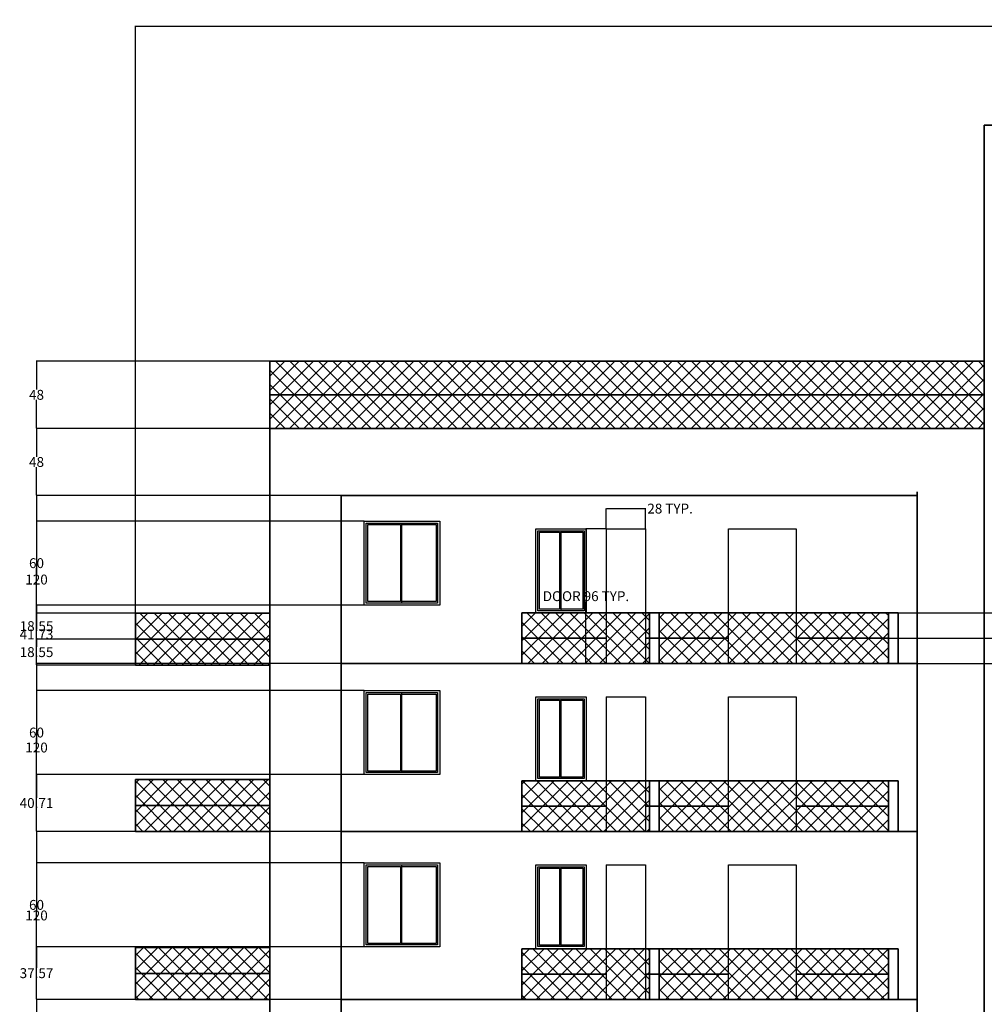
# Model space of a CAD drawing. Units: inches. Extents: x -222 to 1347, y 12 to 1073.
# Tile 2 of 4: x -222 to 467, y 369 to 1073. Entities that reach past the tile are written whole.
import ezdxf

# ---------------------------------------------------------------- set-up
doc = ezdxf.new("R2010")
doc.units = ezdxf.units.IN
doc.header["$MEASUREMENT"] = 0
for name, color, linetype, lineweight in [('A-ANNO-DIMS', 2, 'Continuous', 18), ('A-DOOR', 4, 'Continuous', 25), ('A-ELEV', 7, 'Continuous', 35), ('A-ELEV-PATT', 8, 'Continuous', 13), ('A-GLAZ', 4, 'Continuous', 25)]:
    doc.layers.add(name, color=color, linetype=linetype, lineweight=lineweight)
doc.styles.get("Standard").update_dxf_attribs({"font": 'arial.ttf'})
doc.dimstyles.get("Standard").update_dxf_attribs({"dimtxt": 7.0625, "dimasz": 0.18, "dimexe": 0.18, "dimexo": 0.0625, "dimgap": 0.09, "dimtad": 0, "dimtih": 1, "dimtoh": 1, "dimdec": 4, "dimzin": 0, "dimdsep": 46, "dimlunit": 4, "dimtxsty": 'Standard', "dimcen": 0.09, "dimadec": 0, "dimazin": 0, "dimtfac": 1, "dimtdec": 4, "dimtofl": 0, "dimtmove": 0, "dimatfit": 3, "dimfxl": 1, "dimtolj": 1, "dimtzin": 0, "dimarcsym": 0})

# ---------------------------------------------------------------- blocks, each defined once
blk = doc.blocks.new('*U2')
for p, q in [((1.5, 1.5), (1.5, 58.5)), ((1.5, 58.5), (27, 58.5)), ((27, 1.5), (27, 58.5)), ((27, 58.5), (52.5, 58.5)), ((52.5, 58.5), (52.5, 1.5)), ((27, 1.5), (1.5, 1.5)), ((52.5, 1.5), (27, 1.5))]:
    blk.add_line(p, q)
blk.add_lwpolyline([(0, 0), (0, 60), (54, 60), (54, 0)], close=True)
for points in [[(26, 57.5), (26, 2.5), (2.5, 2.5), (2.5, 57.5), (26, 57.5)], [(27, 57.5), (51.5, 57.5), (51.5, 2.5), (27, 2.5)]]:
    blk.add_lwpolyline(points)
blk = doc.blocks.new('*U3')
for p, q in [((1.5, 1.5), (1.5, 58.5)), ((1.5, 58.5), (18, 58.5)), ((18, 1.5), (18, 58.5)), ((18, 58.5), (34.5, 58.5)), ((34.5, 58.5), (34.5, 1.5)), ((18, 1.5), (1.5, 1.5)), ((34.5, 1.5), (18, 1.5))]:
    blk.add_line(p, q)
blk.add_lwpolyline([(0, 0), (0, 60), (36, 60), (36, 0)], close=True)
for points in [[(17, 57.5), (17, 2.5), (2.5, 2.5), (2.5, 57.5), (17, 57.5)], [(18, 57.5), (33.5, 57.5), (33.5, 2.5), (18, 2.5)]]:
    blk.add_lwpolyline(points)
blk = doc.blocks.new('DOOR-700')
for p, q in [((0, 96.26), (0, 0)), ((0, 96.26), (23.43, 96.26)), ((23.43, 96.26), (28.14, 96.26)), ((28.14, 96.26), (28.14, 0))]:
    blk.add_line(p, q)
blk = doc.blocks.new('DOOR-1200')
for p, q in [((0, 0), (0, 96.26)), ((0, 96.26), (48.21, 96.26)), ((48.21, 96.26), (48.21, 0))]:
    blk.add_line(p, q)
blk = doc.blocks.new('*D6')
at = {"layer": 'A-ANNO-DIMS', "color": 0, "lineweight": -2, "transparency": 16777216}
for p, q in [((197.08, 709.03), (182.52, 709.03)), ((182.7, 708.85), (182.7, 664.64)), ((182.7, 612.95), (182.7, 657.15)), ((197.08, 612.77), (182.52, 612.77))]:
    blk.add_line(p, q, dxfattribs=at)
at = {"layer": 'A-ANNO-DIMS', "color": 0, "transparency": 16777216}
for points in [[(182.67, 708.85), (182.73, 708.85), (182.7, 709.03)], [(182.67, 612.95), (182.73, 612.95), (182.7, 612.77)]]:
    blk.add_solid(points, dxfattribs=at)
at = {"layer": 'Defpoints', "color": 0, "transparency": 16777216}
for p in [(182.7, 709.03), (197.14, 709.03), (197.14, 612.77)]:
    blk.add_point(p, dxfattribs=at)
at = {"layer": 'A-ANNO-DIMS', "color": 0, "transparency": 16777216, "insert": (182.7, 660.9), "char_height": 7.0625, "attachment_point": 5}
blk.add_mtext('\\A1;DOOR 96 TYP.', dxfattribs=at)
blk = doc.blocks.new('*D7')
at = {"layer": 'A-ANNO-DIMS', "color": 0, "lineweight": -2, "transparency": 16777216}
for p, q in [((197.14, 709.09), (197.14, 723.65)), ((197.32, 723.47), (225.1, 723.47)), ((225.28, 709.09), (225.28, 723.65)), ((225.28, 723.47), (225.46, 723.47))]:
    blk.add_line(p, q, dxfattribs=at)
at = {"layer": 'A-ANNO-DIMS', "color": 0, "transparency": 16777216}
for points in [[(197.32, 723.5), (197.32, 723.44), (197.14, 723.47)], [(225.1, 723.5), (225.1, 723.44), (225.28, 723.47)]]:
    blk.add_solid(points, dxfattribs=at)
at = {"layer": 'Defpoints', "color": 0, "transparency": 16777216}
for p in [(225.28, 723.47), (197.14, 709.03), (225.28, 709.03)]:
    blk.add_point(p, dxfattribs=at)
at = {"layer": 'A-ANNO-DIMS', "color": 0, "transparency": 16777216, "insert": (242.8, 723.47), "char_height": 7.0625, "attachment_point": 5}
blk.add_mtext('\\A1;28 TYP.', dxfattribs=at)
blk = doc.blocks.new('*D10')
at = {"layer": 'A-ANNO-DIMS', "color": 0, "lineweight": -2, "transparency": 16777216}
for p, q in [((-139.29, 648.82), (-139.29, 1068.32)), ((-139.11, 1068.14), (546.95, 1068.14)), ((1261.84, 1068.14), (575.78, 1068.14)), ((1262.02, 648.82), (1262.02, 1068.32))]:
    blk.add_line(p, q, dxfattribs=at)
at = {"layer": 'A-ANNO-DIMS', "color": 0, "transparency": 16777216}
for points in [[(-139.11, 1068.17), (-139.11, 1068.11), (-139.29, 1068.14)], [(1261.84, 1068.17), (1261.84, 1068.11), (1262.02, 1068.14)]]:
    blk.add_solid(points, dxfattribs=at)
at = {"layer": 'Defpoints', "color": 0, "transparency": 16777216}
for p in [(1262.02, 1068.14), (-139.29, 648.76), (1262.02, 648.76)]:
    blk.add_point(p, dxfattribs=at)
at = {"layer": 'A-ANNO-DIMS', "color": 0, "transparency": 16777216, "insert": (561.37, 1068.14), "char_height": 7.062, "attachment_point": 5}
blk.add_mtext('\\A1;1401.3', dxfattribs=at)
blk = doc.blocks.new('*D42')
at = {"layer": 'A-ANNO-DIMS', "color": 0, "lineweight": -2, "transparency": 16777216}
for p, q in [((7.74, 372.77), (-210.12, 372.77)), ((-209.94, 372.59), (-209.94, 353.91)), ((-209.94, 327.84), (-209.94, 346.52)), ((7.74, 327.66), (-210.12, 327.66))]:
    blk.add_line(p, q, dxfattribs=at)
at = {"layer": 'A-ANNO-DIMS', "color": 0, "transparency": 16777216}
for points in [[(-209.97, 372.59), (-209.91, 372.59), (-209.94, 372.77)], [(-209.97, 327.84), (-209.91, 327.84), (-209.94, 327.66)]]:
    blk.add_solid(points, dxfattribs=at)
at = {"layer": 'Defpoints', "color": 0, "transparency": 16777216}
for p in [(-209.94, 372.77), (7.81, 372.77), (7.81, 327.66)]:
    blk.add_point(p, dxfattribs=at)
at = {"layer": 'A-ANNO-DIMS', "color": 0, "transparency": 16777216, "insert": (-209.94, 350.21), "char_height": 7.062, "attachment_point": 5}
blk.add_mtext('\\A1;45.1', dxfattribs=at)
blk = doc.blocks.new('*D43')
at = {"layer": 'A-ANNO-DIMS', "color": 0, "lineweight": -2, "transparency": 16777216}
for p, q in [((7.74, 492.77), (-210.12, 492.77)), ((-209.94, 492.59), (-209.94, 436.46)), ((-209.94, 372.95), (-209.94, 429.07)), ((7.74, 372.77), (-210.12, 372.77))]:
    blk.add_line(p, q, dxfattribs=at)
at = {"layer": 'A-ANNO-DIMS', "color": 0, "transparency": 16777216}
for points in [[(-209.97, 492.59), (-209.91, 492.59), (-209.94, 492.77)], [(-209.97, 372.95), (-209.91, 372.95), (-209.94, 372.77)]]:
    blk.add_solid(points, dxfattribs=at)
at = {"layer": 'Defpoints', "color": 0, "transparency": 16777216}
for p in [(-209.94, 492.77), (7.81, 492.77), (7.81, 372.77)]:
    blk.add_point(p, dxfattribs=at)
at = {"layer": 'A-ANNO-DIMS', "color": 0, "transparency": 16777216, "insert": (-209.94, 432.77), "char_height": 7.062, "attachment_point": 5}
blk.add_mtext('\\A1;120', dxfattribs=at)
blk = doc.blocks.new('*D44')
at = {"layer": 'A-ANNO-DIMS', "color": 0, "lineweight": -2, "transparency": 16777216}
for p, q in [((7.74, 612.77), (-210.12, 612.77)), ((-209.94, 612.59), (-209.94, 556.46)), ((-209.94, 492.95), (-209.94, 549.07)), ((7.74, 492.77), (-210.12, 492.77))]:
    blk.add_line(p, q, dxfattribs=at)
at = {"layer": 'A-ANNO-DIMS', "color": 0, "transparency": 16777216}
for points in [[(-209.97, 612.59), (-209.91, 612.59), (-209.94, 612.77)], [(-209.97, 492.95), (-209.91, 492.95), (-209.94, 492.77)]]:
    blk.add_solid(points, dxfattribs=at)
at = {"layer": 'Defpoints', "color": 0, "transparency": 16777216}
for p in [(-209.94, 612.77), (7.81, 612.77), (7.81, 492.77)]:
    blk.add_point(p, dxfattribs=at)
at = {"layer": 'A-ANNO-DIMS', "color": 0, "transparency": 16777216, "insert": (-209.94, 552.77), "char_height": 7.062, "attachment_point": 5}
blk.add_mtext('\\A1;120', dxfattribs=at)
blk = doc.blocks.new('*D45')
at = {"layer": 'A-ANNO-DIMS', "color": 0, "lineweight": -2, "transparency": 16777216}
for p, q in [((7.74, 732.77), (-210.12, 732.77)), ((-209.94, 732.59), (-209.94, 676.46)), ((-209.94, 612.95), (-209.94, 669.07)), ((7.74, 612.77), (-210.12, 612.77))]:
    blk.add_line(p, q, dxfattribs=at)
at = {"layer": 'A-ANNO-DIMS', "color": 0, "transparency": 16777216}
for points in [[(-209.97, 732.59), (-209.91, 732.59), (-209.94, 732.77)], [(-209.97, 612.95), (-209.91, 612.95), (-209.94, 612.77)]]:
    blk.add_solid(points, dxfattribs=at)
at = {"layer": 'Defpoints', "color": 0, "transparency": 16777216}
for p in [(-209.94, 732.77), (7.81, 732.77), (7.81, 612.77)]:
    blk.add_point(p, dxfattribs=at)
at = {"layer": 'A-ANNO-DIMS', "color": 0, "transparency": 16777216, "insert": (-209.94, 672.77), "char_height": 7.062, "attachment_point": 5}
blk.add_mtext('\\A1;120', dxfattribs=at)
blk = doc.blocks.new('*D46')
at = {"layer": 'A-ANNO-DIMS', "color": 0, "lineweight": -2, "transparency": 16777216}
for p, q in [((-43.22, 780.77), (-210.12, 780.77)), ((-209.94, 780.59), (-209.94, 760.46)), ((-209.94, 732.95), (-209.94, 753.07)), ((7.74, 732.77), (-210.12, 732.77))]:
    blk.add_line(p, q, dxfattribs=at)
at = {"layer": 'A-ANNO-DIMS', "color": 0, "transparency": 16777216}
for points in [[(-209.97, 780.59), (-209.91, 780.59), (-209.94, 780.77)], [(-209.97, 732.95), (-209.91, 732.95), (-209.94, 732.77)]]:
    blk.add_solid(points, dxfattribs=at)
at = {"layer": 'Defpoints', "color": 0, "transparency": 16777216}
for p in [(-209.94, 780.77), (-43.16, 780.77), (7.81, 732.77)]:
    blk.add_point(p, dxfattribs=at)
at = {"layer": 'A-ANNO-DIMS', "color": 0, "transparency": 16777216, "insert": (-209.94, 756.77), "char_height": 7.062, "attachment_point": 5}
blk.add_mtext('\\A1;48', dxfattribs=at)
blk = doc.blocks.new('*D47')
at = {"layer": 'A-ANNO-DIMS', "color": 0, "lineweight": -2, "transparency": 16777216}
for p, q in [((-43.22, 828.77), (-210.12, 828.77)), ((-209.94, 828.59), (-209.94, 808.46)), ((-209.94, 780.95), (-209.94, 801.07)), ((-43.22, 780.77), (-210.12, 780.77))]:
    blk.add_line(p, q, dxfattribs=at)
at = {"layer": 'A-ANNO-DIMS', "color": 0, "transparency": 16777216}
for points in [[(-209.97, 828.59), (-209.91, 828.59), (-209.94, 828.77)], [(-209.97, 780.95), (-209.91, 780.95), (-209.94, 780.77)]]:
    blk.add_solid(points, dxfattribs=at)
at = {"layer": 'Defpoints', "color": 0, "transparency": 16777216}
for p in [(-209.94, 828.77), (-43.16, 828.77), (-43.16, 780.77)]:
    blk.add_point(p, dxfattribs=at)
at = {"layer": 'A-ANNO-DIMS', "color": 0, "transparency": 16777216, "insert": (-209.94, 804.77), "char_height": 7.062, "attachment_point": 5}
blk.add_mtext('\\A1;48', dxfattribs=at)
blk = doc.blocks.new('*D50')
at = {"layer": 'A-ANNO-DIMS', "color": 0, "lineweight": -2, "transparency": 16777216}
for p, q in [((24.14, 410.34), (-210.12, 410.34)), ((-209.94, 410.16), (-209.94, 395.25)), ((-209.94, 372.95), (-209.94, 387.85)), ((136.83, 372.77), (-210.12, 372.77))]:
    blk.add_line(p, q, dxfattribs=at)
at = {"layer": 'A-ANNO-DIMS', "color": 0, "transparency": 16777216}
for points in [[(-209.97, 410.16), (-209.91, 410.16), (-209.94, 410.34)], [(-209.97, 372.95), (-209.91, 372.95), (-209.94, 372.77)]]:
    blk.add_solid(points, dxfattribs=at)
at = {"layer": 'Defpoints', "color": 0, "transparency": 16777216}
for p in [(-209.94, 410.34), (24.2, 410.34), (136.89, 372.77)]:
    blk.add_point(p, dxfattribs=at)
at = {"layer": 'A-ANNO-DIMS', "color": 0, "transparency": 16777216, "insert": (-209.94, 391.55), "char_height": 7.062, "attachment_point": 5}
blk.add_mtext('\\A1;37.57', dxfattribs=at)
blk = doc.blocks.new('*D51')
at = {"layer": 'A-ANNO-DIMS', "color": 0, "lineweight": -2, "transparency": 16777216}
for p, q in [((24.14, 470.34), (-210.12, 470.34)), ((-209.94, 470.16), (-209.94, 444.03)), ((-209.94, 410.52), (-209.94, 436.64)), ((24.14, 410.34), (-210.12, 410.34))]:
    blk.add_line(p, q, dxfattribs=at)
at = {"layer": 'A-ANNO-DIMS', "color": 0, "transparency": 16777216}
for points in [[(-209.97, 470.16), (-209.91, 470.16), (-209.94, 470.34)], [(-209.97, 410.52), (-209.91, 410.52), (-209.94, 410.34)]]:
    blk.add_solid(points, dxfattribs=at)
at = {"layer": 'Defpoints', "color": 0, "transparency": 16777216}
for p in [(-209.94, 470.34), (24.2, 470.34), (24.2, 410.34)]:
    blk.add_point(p, dxfattribs=at)
at = {"layer": 'A-ANNO-DIMS', "color": 0, "transparency": 16777216, "insert": (-209.94, 440.34), "char_height": 7.062, "attachment_point": 5}
blk.add_mtext('\\A1;60', dxfattribs=at)
blk = doc.blocks.new('*D52')
at = {"layer": 'A-ANNO-DIMS', "color": 0, "lineweight": -2, "transparency": 16777216}
for p, q in [((24.14, 533.47), (-210.12, 533.47)), ((-209.94, 533.29), (-209.94, 516.82)), ((-209.94, 492.95), (-209.94, 509.42)), ((136.83, 492.77), (-210.12, 492.77))]:
    blk.add_line(p, q, dxfattribs=at)
at = {"layer": 'A-ANNO-DIMS', "color": 0, "transparency": 16777216}
for points in [[(-209.97, 533.29), (-209.91, 533.29), (-209.94, 533.47)], [(-209.97, 492.95), (-209.91, 492.95), (-209.94, 492.77)]]:
    blk.add_solid(points, dxfattribs=at)
at = {"layer": 'Defpoints', "color": 0, "transparency": 16777216}
for p in [(-209.94, 533.47), (24.2, 533.47), (136.89, 492.77)]:
    blk.add_point(p, dxfattribs=at)
at = {"layer": 'A-ANNO-DIMS', "color": 0, "transparency": 16777216, "insert": (-209.94, 513.12), "char_height": 7.062, "attachment_point": 5}
blk.add_mtext('\\A1;40.71', dxfattribs=at)
blk = doc.blocks.new('*D53')
at = {"layer": 'A-ANNO-DIMS', "color": 0, "lineweight": -2, "transparency": 16777216}
for p, q in [((24.14, 593.47), (-210.12, 593.47)), ((-209.94, 593.29), (-209.94, 567.17)), ((-209.94, 533.65), (-209.94, 559.78)), ((24.14, 533.47), (-210.12, 533.47))]:
    blk.add_line(p, q, dxfattribs=at)
at = {"layer": 'A-ANNO-DIMS', "color": 0, "transparency": 16777216}
for points in [[(-209.97, 593.29), (-209.91, 593.29), (-209.94, 593.47)], [(-209.97, 533.65), (-209.91, 533.65), (-209.94, 533.47)]]:
    blk.add_solid(points, dxfattribs=at)
at = {"layer": 'Defpoints', "color": 0, "transparency": 16777216}
for p in [(-209.94, 593.47), (24.2, 593.47), (24.2, 533.47)]:
    blk.add_point(p, dxfattribs=at)
at = {"layer": 'A-ANNO-DIMS', "color": 0, "transparency": 16777216, "insert": (-209.94, 563.47), "char_height": 7.062, "attachment_point": 5}
blk.add_mtext('\\A1;60', dxfattribs=at)
blk = doc.blocks.new('*D54')
at = {"layer": 'A-ANNO-DIMS', "color": 0, "lineweight": -2, "transparency": 16777216}
for p, q in [((24.14, 654.5), (-210.12, 654.5)), ((-209.94, 654.32), (-209.94, 637.33)), ((-209.94, 612.95), (-209.94, 629.93)), ((136.83, 612.77), (-210.12, 612.77))]:
    blk.add_line(p, q, dxfattribs=at)
at = {"layer": 'A-ANNO-DIMS', "color": 0, "transparency": 16777216}
for points in [[(-209.97, 654.32), (-209.91, 654.32), (-209.94, 654.5)], [(-209.97, 612.95), (-209.91, 612.95), (-209.94, 612.77)]]:
    blk.add_solid(points, dxfattribs=at)
at = {"layer": 'Defpoints', "color": 0, "transparency": 16777216}
for p in [(-209.94, 654.5), (24.2, 654.5), (136.89, 612.77)]:
    blk.add_point(p, dxfattribs=at)
at = {"layer": 'A-ANNO-DIMS', "color": 0, "transparency": 16777216, "insert": (-209.94, 633.63), "char_height": 7.062, "attachment_point": 5}
blk.add_mtext('\\A1;41.73', dxfattribs=at)
blk = doc.blocks.new('*D55')
at = {"layer": 'A-ANNO-DIMS', "color": 0, "lineweight": -2, "transparency": 16777216}
for p, q in [((24.14, 714.5), (-210.12, 714.5)), ((-209.94, 714.32), (-209.94, 688.19)), ((-209.94, 654.68), (-209.94, 680.8)), ((24.14, 654.5), (-210.12, 654.5))]:
    blk.add_line(p, q, dxfattribs=at)
at = {"layer": 'A-ANNO-DIMS', "color": 0, "transparency": 16777216}
for points in [[(-209.97, 714.32), (-209.91, 714.32), (-209.94, 714.5)], [(-209.97, 654.68), (-209.91, 654.68), (-209.94, 654.5)]]:
    blk.add_solid(points, dxfattribs=at)
at = {"layer": 'Defpoints', "color": 0, "transparency": 16777216}
for p in [(-209.94, 714.5), (24.2, 714.5), (24.2, 654.5)]:
    blk.add_point(p, dxfattribs=at)
at = {"layer": 'A-ANNO-DIMS', "color": 0, "transparency": 16777216, "insert": (-209.94, 684.5), "char_height": 7.062, "attachment_point": 5}
blk.add_mtext('\\A1;60', dxfattribs=at)
blk = doc.blocks.new('*D56')
at = {"layer": 'A-ANNO-DIMS', "color": 0, "lineweight": -2, "transparency": 16777216}
for p, q in [((-139.35, 630.21), (-210.12, 630.21)), ((-209.94, 630.03), (-209.94, 624.63)), ((-209.94, 611.84), (-209.94, 617.24)), ((-139.35, 611.66), (-210.12, 611.66))]:
    blk.add_line(p, q, dxfattribs=at)
at = {"layer": 'A-ANNO-DIMS', "color": 0, "transparency": 16777216}
for points in [[(-209.97, 630.03), (-209.91, 630.03), (-209.94, 630.21)], [(-209.97, 611.84), (-209.91, 611.84), (-209.94, 611.66)]]:
    blk.add_solid(points, dxfattribs=at)
at = {"layer": 'Defpoints', "color": 0, "transparency": 16777216}
for p in [(-209.94, 630.21), (-139.29, 630.21), (-139.29, 611.66)]:
    blk.add_point(p, dxfattribs=at)
at = {"layer": 'A-ANNO-DIMS', "color": 0, "transparency": 16777216, "insert": (-209.94, 620.93), "char_height": 7.062, "attachment_point": 5}
blk.add_mtext('\\A1;18.55', dxfattribs=at)
blk = doc.blocks.new('*D57')
at = {"layer": 'A-ANNO-DIMS', "color": 0, "lineweight": -2, "transparency": 16777216}
for p, q in [((-139.35, 648.76), (-210.12, 648.76)), ((-209.94, 648.58), (-209.94, 643.18)), ((-209.94, 630.39), (-209.94, 635.79)), ((-139.35, 630.21), (-210.12, 630.21))]:
    blk.add_line(p, q, dxfattribs=at)
at = {"layer": 'A-ANNO-DIMS', "color": 0, "transparency": 16777216}
for points in [[(-209.97, 648.58), (-209.91, 648.58), (-209.94, 648.76)], [(-209.97, 630.39), (-209.91, 630.39), (-209.94, 630.21)]]:
    blk.add_solid(points, dxfattribs=at)
at = {"layer": 'Defpoints', "color": 0, "transparency": 16777216}
for p in [(-209.94, 648.76), (-139.29, 648.76), (-139.29, 630.21)]:
    blk.add_point(p, dxfattribs=at)
at = {"layer": 'A-ANNO-DIMS', "color": 0, "transparency": 16777216, "insert": (-209.94, 639.48), "char_height": 7.062, "attachment_point": 5}
blk.add_mtext('\\A1;18.55', dxfattribs=at)
blk = doc.blocks.new('*D68')
at = {"layer": 'A-ANNO-DIMS', "color": 0, "lineweight": -2, "transparency": 16777216}
for p, q in [((398.84, 630.9), (1332.85, 630.9)), ((1332.67, 630.72), (1332.67, 625.53)), ((405.84, 612.77), (1332.85, 612.77)), ((1332.67, 612.95), (1332.67, 618.13))]:
    blk.add_line(p, q, dxfattribs=at)
at = {"layer": 'A-ANNO-DIMS', "color": 0, "transparency": 16777216}
for points in [[(1332.64, 630.72), (1332.7, 630.72), (1332.67, 630.9)], [(1332.64, 612.95), (1332.7, 612.95), (1332.67, 612.77)]]:
    blk.add_solid(points, dxfattribs=at)
at = {"layer": 'Defpoints', "color": 0, "transparency": 16777216}
for p in [(398.78, 630.9), (1332.67, 630.9), (405.78, 612.77)]:
    blk.add_point(p, dxfattribs=at)
at = {"layer": 'A-ANNO-DIMS', "color": 0, "transparency": 16777216, "insert": (1332.67, 621.83), "char_height": 7.062, "attachment_point": 5}
blk.add_mtext('\\A1;18.13', dxfattribs=at)
blk = doc.blocks.new('*D69')
at = {"layer": 'A-ANNO-DIMS', "color": 0, "lineweight": -2, "transparency": 16777216}
for p, q in [((405.84, 649.03), (1332.85, 649.03)), ((1332.67, 648.85), (1332.67, 643.66)), ((1332.67, 631.08), (1332.67, 636.26)), ((398.84, 630.9), (1332.85, 630.9))]:
    blk.add_line(p, q, dxfattribs=at)
at = {"layer": 'A-ANNO-DIMS', "color": 0, "transparency": 16777216}
for points in [[(1332.64, 648.85), (1332.7, 648.85), (1332.67, 649.03)], [(1332.64, 631.08), (1332.7, 631.08), (1332.67, 630.9)]]:
    blk.add_solid(points, dxfattribs=at)
at = {"layer": 'Defpoints', "color": 0, "transparency": 16777216}
for p in [(405.78, 649.03), (1332.67, 649.03), (398.78, 630.9)]:
    blk.add_point(p, dxfattribs=at)
at = {"layer": 'A-ANNO-DIMS', "color": 0, "transparency": 16777216, "insert": (1332.67, 639.96), "char_height": 7.062, "attachment_point": 5}
blk.add_mtext('\\A1;18.13', dxfattribs=at)

msp = doc.modelspace()

# ---------------------------------------------------------------- hatches: boundary and pattern name
at = {"layer": 'A-ELEV-PATT'}
h = msp.add_hatch(dxfattribs=at)
h.set_pattern_fill('ANSI37', color=256, scale=58)
h.paths.add_polyline_path([(467.3436, 828.7653), (-43.1601, 828.7653), (-43.1601, 804.7653), (467.3436, 804.7653)])
h.paths.add_polyline_path([(467.3436, 804.7653), (-43.1601, 804.7653), (-43.1601, 780.7653), (192.0309, 780.7653), (467.3436, 780.7653)])
h = msp.add_hatch(dxfattribs=at)
h.set_pattern_fill('ANSI37', color=256, scale=58)
h.paths.add_polyline_path([(-43.1601, 648.7576), (-139.2916, 648.7576), (-139.2916, 630.2077), (-43.1601, 630.2077)])
h.paths.add_polyline_path([(-43.1601, 630.2077), (-139.2916, 630.2077), (-139.2916, 611.6578), (-43.1601, 611.6578)])
h.paths.add_polyline_path([(-43.1601, 529.8651), (-139.2916, 529.8651), (-139.2916, 511.3152), (-43.1601, 511.3152)])
h.paths.add_polyline_path([(-43.1601, 511.3152), (-139.2916, 511.3152), (-139.2916, 492.7653), (-43.1601, 492.7653)])
h.paths.add_polyline_path([(-43.1601, 409.8651), (-139.2916, 409.8651), (-139.2916, 391.3152), (-43.1601, 391.3152)])
h.paths.add_polyline_path([(-43.1601, 391.3152), (-139.2916, 391.3152), (-139.2916, 372.7653), (-43.1601, 372.7653)])
h.paths.add_polyline_path([(-43.1601, 244.764), (-139.2916, 244.764), (-139.2916, 226.2141), (-43.1601, 226.2141)])
h.paths.add_polyline_path([(-43.1601, 226.2141), (-139.2916, 226.2141), (-139.2916, 207.6642), (-43.1601, 207.6642)])
h = msp.add_hatch(dxfattribs=at)
h.set_pattern_fill('ANSI37', color=256, scale=58)
h.paths.add_polyline_path([(197.1405, 649.0276), (146.8914, 649.0276), (136.8908, 649.0276), (136.8908, 630.8964), (197.1405, 630.8964)])
h.paths.add_polyline_path([(197.1405, 630.8964), (136.8908, 630.8964), (136.8908, 612.7653), (197.1405, 612.7653)])
h.paths.add_polyline_path([(225.2842, 649.0276), (197.1405, 649.0276), (197.1405, 630.8964), (197.1405, 612.7653), (225.2842, 612.7653)])
h.paths.add_polyline_path([(228.1006, 649.0276), (225.2842, 649.0276), (225.2842, 630.8964), (228.1006, 630.8964)])
h.paths.add_polyline_path([(228.1006, 630.8964), (225.2842, 630.8964), (225.2842, 612.7653), (228.1006, 612.7653)])
h.paths.add_polyline_path([(284.6018, 649.0276), (235.1006, 649.0276), (235.1006, 630.8964), (284.6018, 630.8964)])
h.paths.add_polyline_path([(284.6018, 630.8964), (235.1006, 630.8964), (235.1006, 612.7653), (284.6018, 612.7653)])
h.paths.add_polyline_path([(332.8148, 649.0276), (284.6018, 649.0276), (284.6018, 612.7653), (332.8148, 612.7653)])
h.paths.add_polyline_path([(398.776, 649.0276), (332.8148, 649.0276), (332.8148, 630.8964), (398.776, 630.8964)])
h.paths.add_polyline_path([(398.776, 630.8964), (332.8148, 630.8964), (332.8148, 612.7653), (398.776, 612.7653)])
h.paths.add_polyline_path([(197.1405, 529.0276), (146.8914, 529.0276), (136.8908, 529.0276), (136.8908, 510.8964), (197.1405, 510.8964)])
h.paths.add_polyline_path([(197.1405, 510.8964), (136.8908, 510.8964), (136.8908, 492.7653), (197.1405, 492.7653)])
h.paths.add_polyline_path([(228.1006, 529.0276), (225.2842, 529.0276), (225.2842, 510.9211), (228.1006, 510.9211)])
h.paths.add_polyline_path([(228.1006, 510.9211), (225.2842, 510.9211), (225.2842, 492.7653), (228.1006, 492.7653)])
h.paths.add_polyline_path([(284.6018, 529.0276), (235.1006, 529.0276), (235.1006, 510.9211), (284.6018, 510.9211)])
h.paths.add_polyline_path([(284.6018, 510.9211), (235.1006, 510.9211), (235.1006, 492.7653), (284.6018, 492.7653)])
h.paths.add_polyline_path([(332.8148, 529.0276), (284.6018, 529.0276), (284.6018, 510.9211), (284.6018, 492.7653), (332.8148, 492.7653)])
h.paths.add_polyline_path([(398.776, 529.0276), (332.8148, 529.0276), (332.8148, 510.9211), (398.776, 510.9211)])
h.paths.add_polyline_path([(398.776, 510.9211), (332.8148, 510.9211), (332.8148, 492.7653), (398.776, 492.7653)])
h.paths.add_polyline_path([(398.776, 409.0276), (332.8148, 409.0276), (332.8148, 390.8964), (398.776, 390.8964)])
h.paths.add_polyline_path([(398.776, 390.8964), (332.8148, 390.8964), (332.8148, 372.7653), (398.776, 372.7653)])
h.paths.add_polyline_path([(284.6018, 409.0276), (235.1006, 409.0276), (235.1006, 390.8964), (284.6018, 390.8964)])
h.paths.add_polyline_path([(332.8148, 409.0276), (284.6018, 409.0276), (284.6018, 390.8964), (284.6018, 372.7653), (332.8148, 372.7653), (332.8148, 390.8964)])
h.paths.add_polyline_path([(284.6018, 390.8964), (235.1006, 390.8964), (235.1006, 372.7653), (284.6018, 372.7653)])
h.paths.add_polyline_path([(228.1006, 409.0276), (225.2842, 409.0276), (225.2842, 390.8964), (228.1006, 390.8964)])
h.paths.add_polyline_path([(228.1006, 390.8964), (225.2842, 390.8964), (225.2842, 372.7653), (228.1006, 372.7653)])
h.paths.add_polyline_path([(197.1405, 409.0276), (146.8914, 409.0276), (136.8908, 409.0276), (136.8908, 390.8964), (197.1405, 390.8964)])
h.paths.add_polyline_path([(197.1405, 390.8964), (136.8908, 390.8964), (136.8908, 372.7653), (197.1405, 372.7653)])
h = msp.add_hatch(dxfattribs=at)
h.set_pattern_fill('ANSI37', color=256, scale=58)
h.paths.add_polyline_path([(925.5902, 529.0276), (897.4464, 529.0276), (897.4464, 492.7653), (925.5902, 492.7653)])
h.paths.add_polyline_path([(925.5902, 409.0276), (897.4464, 409.0276), (897.4464, 372.7653), (925.5902, 372.7653)])
h.paths.add_polyline_path([(225.2842, 409.0276), (197.1405, 409.0276), (197.1405, 372.7653), (225.2842, 372.7653)])
h.paths.add_polyline_path([(225.2842, 529.0276), (197.1405, 529.0276), (197.1405, 492.7653), (225.2842, 492.7653)])

# ---------------------------------------------------------------- linework, layer by layer
at = {"layer": 'A-ELEV'}
for p, q in [((467.3436, 828.7653), (467.3436, 997.488)), ((467.3436, 997.488), (655.387, 997.488)), ((-43.1601, 780.7653), (-43.1601, 828.7653)), ((-43.1601, 828.7653), (467.3436, 828.7653)), ((467.3436, 828.7653), (467.3436, 780.7653)), ((-43.1601, 804.7653), (467.3436, 804.7653)), ((-43.1601, 207.6642), (-43.1601, 780.7653)), ((192.0309, 780.7653), (-43.1601, 780.7653)), ((192.0309, 780.7653), (467.3436, 780.7653)), ((467.3436, 87.6642), (467.3436, 780.7653)), ((7.8066, 732.7653), (419.3436, 732.7653)), ((7.8066, 732.7653), (7.8066, 656.5028)), ((419.3436, 447.6642), (419.3436, 735.4477)), ((7.8066, 584.7569), (7.8066, 656.5028)), ((-43.1601, 648.7576), (-139.2916, 648.7576)), ((-139.2916, 648.7576), (-139.2916, 611.6578)), ((136.8908, 612.7653), (136.8908, 649.0276)), ((136.8908, 649.0276), (146.8914, 649.0276)), ((146.8914, 649.0276), (398.776, 649.0276)), ((228.1006, 612.7653), (228.1006, 649.0276)), ((235.1006, 612.7653), (235.1006, 649.0276)), ((398.776, 649.0276), (398.776, 612.7653)), ((405.776, 649.0276), (398.776, 649.0276)), ((405.776, 612.7653), (405.776, 649.0276)), ((-139.2916, 630.2077), (-43.1601, 630.2077)), ((136.8908, 630.8964), (197.1405, 630.8964)), ((225.2842, 630.8964), (284.6018, 630.8964)), ((332.8148, 630.8964), (398.776, 630.8964)), ((7.8066, 612.7653), (419.3436, 612.7653)), ((-43.1601, 611.6578), (-139.2916, 611.6578)), ((7.8066, 584.7569), (7.8066, 347.9663)), ((-43.1601, 529.8651), (-139.2916, 529.8651)), ((-139.2916, 529.8651), (-139.2916, 492.7653)), ((136.8908, 492.7653), (136.8908, 529.0276)), ((136.8908, 529.0276), (146.8914, 529.0276)), ((146.8914, 529.0276), (398.776, 529.0276)), ((228.1006, 492.7653), (228.1006, 529.0276)), ((235.1006, 492.7653), (235.1006, 529.0276)), ((398.776, 529.0276), (398.776, 492.7653)), ((405.776, 529.0276), (398.776, 529.0276)), ((405.776, 492.7653), (405.776, 529.0276)), ((-139.2916, 511.3152), (-43.1601, 511.3152)), ((136.8908, 510.8964), (197.1405, 510.8964)), ((225.2842, 510.9211), (284.6018, 510.9211)), ((332.8148, 510.9211), (398.776, 510.9211)), ((-43.1601, 492.7653), (-139.2916, 492.7653)), ((7.8066, 492.7653), (419.3436, 492.7653)), ((419.3436, 447.6642), (419.3436, 327.6642)), ((-43.1601, 409.8651), (-139.2916, 409.8651)), ((-139.2916, 409.8651), (-139.2916, 372.7653)), ((136.8908, 372.7653), (136.8908, 409.0276)), ((136.8908, 409.0276), (146.8914, 409.0276)), ((146.8914, 409.0276), (398.776, 409.0276)), ((228.1006, 372.7653), (228.1006, 409.0276)), ((235.1006, 372.7653), (235.1006, 409.0276)), ((398.776, 409.0276), (398.776, 372.7653)), ((405.776, 409.0276), (398.776, 409.0276)), ((405.776, 372.7653), (405.776, 409.0276)), ((-139.2916, 391.3152), (-43.1601, 391.3152)), ((136.8908, 390.8964), (197.1405, 390.8964)), ((225.2842, 390.8964), (284.6018, 390.8964)), ((332.8148, 390.8964), (398.776, 390.8964)), ((-43.1601, 372.7653), (-139.2916, 372.7653)), ((7.8066, 372.7653), (419.3436, 372.7653))]:
    msp.add_line(p, q, dxfattribs=at)

# ---------------------------------------------------------------- block references
at = {"layer": 'A-DOOR'}
for name, p in [('DOOR-700', (197.14, 612.7651)), ('DOOR-1200', (284.602, 612.7651)), ('DOOR-700', (197.14, 492.7651)), ('DOOR-1200', (284.602, 492.7651)), ('DOOR-700', (197.14, 372.7651)), ('DOOR-1200', (284.602, 372.7651))]:
    msp.add_blockref(name, p, dxfattribs=at)
at = {"layer": 'A-GLAZ'}
for name, p in [('*U2', (24.1991, 654.4958)), ('*U3', (146.8914, 649.0276)), ('*U2', (24.1991, 533.4746)), ('*U3', (146.8914, 529.0276)), ('*U2', (24.1991, 410.3378)), ('*U3', (146.8914, 409.0276))]:
    msp.add_blockref(name, p, dxfattribs=at)

# ---------------------------------------------------------------- dimensions: what is measured, and where the dimension line sits
at = {"layer": 'A-ANNO-DIMS'}
dim = msp.add_linear_dim(base=(1262.0222, 1068.138), p1=(-139.2916, 648.7576), p2=(1262.0222, 648.7576), dimstyle='Standard', override={"dimdec": 1, "dimlfac": 1, "dimrnd": 0, "dimzin": 0, "dimdsep": 46, "dimlunit": 2}, dxfattribs=at)
dim.commit()
dim.dimension.update_dxf_attribs({"geometry": '*D10', "text_midpoint": (561.3653, 1068.138)})
for base, p1, p2, override, picture, middle in [((-209.9416, 828.7653), (-43.1601, 780.7653), (-43.1601, 828.7653), {"dimdec": 0, "dimlfac": 1, "dimrnd": 0, "dimzin": 0, "dimdsep": 46, "dimlunit": 2}, '*D47', (-209.9416, 804.7653)), ((-209.9416, 780.7653), (7.8066, 732.7653), (-43.1601, 780.7653), {"dimdec": 0, "dimlfac": 1, "dimrnd": 0, "dimzin": 0, "dimdsep": 46, "dimlunit": 2}, '*D46', (-209.9416, 756.7653)), ((-209.9416, 732.7653), (7.8066, 612.7653), (7.8066, 732.7653), {"dimdec": 0, "dimlfac": 1, "dimrnd": 0, "dimzin": 0, "dimdsep": 46, "dimlunit": 2}, '*D45', (-209.9416, 672.7653)), ((-209.9416, 714.4958), (24.1991, 654.4958), (24.1991, 714.4958), {"dimdec": 0, "dimlfac": 1, "dimrnd": 0, "dimzin": 0, "dimdsep": 46, "dimlunit": 2}, '*D55', (-209.9416, 684.4958)), ((-209.9416, 654.4958), (136.8908, 612.7653), (24.1991, 654.4958), {"dimdec": 2, "dimlfac": 1, "dimrnd": 0, "dimzin": 0, "dimdsep": 46, "dimlunit": 2}, '*D54', (-209.9416, 633.6306)), ((-209.9416, 648.7576), (-139.2916, 630.2077), (-139.2916, 648.7576), {"dimdec": 2, "dimlfac": 1, "dimrnd": 0, "dimzin": 0, "dimdsep": 46, "dimlunit": 2}, '*D57', (-209.9416, 639.4827)), ((1332.6722, 649.0276), (398.776, 630.8964), (405.776, 649.0276), {"dimdec": 2, "dimlfac": 1, "dimrnd": 0, "dimzin": 0, "dimdsep": 46, "dimlunit": 2}, '*D69', (1332.6722, 639.962)), ((-209.9416, 630.2077), (-139.2916, 611.6578), (-139.2916, 630.2077), {"dimdec": 2, "dimlfac": 1, "dimrnd": 0, "dimzin": 0, "dimdsep": 46, "dimlunit": 2}, '*D56', (-209.9416, 620.9328)), ((1332.6722, 630.8964), (405.776, 612.7653), (398.776, 630.8964), {"dimdec": 2, "dimlfac": 1, "dimrnd": 0, "dimzin": 0, "dimdsep": 46, "dimlunit": 2}, '*D68', (1332.6722, 621.8309)), ((-209.9416, 612.7653), (7.8066, 492.7653), (7.8066, 612.7653), {"dimdec": 0, "dimlfac": 1, "dimrnd": 0, "dimzin": 0, "dimdsep": 46, "dimlunit": 2}, '*D44', (-209.9416, 552.7653)), ((-209.9416, 593.4746), (24.1991, 533.4746), (24.1991, 593.4746), {"dimdec": 0, "dimlfac": 1, "dimrnd": 0, "dimzin": 0, "dimdsep": 46, "dimlunit": 2}, '*D53', (-209.9416, 563.4746)), ((-209.9416, 533.4746), (136.8908, 492.7653), (24.1991, 533.4746), {"dimdec": 2, "dimlfac": 1, "dimrnd": 0, "dimzin": 0, "dimdsep": 46, "dimlunit": 2}, '*D52', (-209.9416, 513.12)), ((-209.9416, 492.7653), (7.8066, 372.7653), (7.8066, 492.7653), {"dimdec": 0, "dimlfac": 1, "dimrnd": 0, "dimzin": 0, "dimdsep": 46, "dimlunit": 2}, '*D43', (-209.9416, 432.7653)), ((-209.9416, 470.3378), (24.1991, 410.3378), (24.1991, 470.3378), {"dimdec": 0, "dimlfac": 1, "dimrnd": 0, "dimzin": 0, "dimdsep": 46, "dimlunit": 2}, '*D51', (-209.9416, 440.3378)), ((-209.9416, 410.3378), (136.8908, 372.7653), (24.1991, 410.3378), {"dimdec": 2, "dimlfac": 1, "dimrnd": 0, "dimzin": 0, "dimdsep": 46, "dimlunit": 2}, '*D50', (-209.9416, 391.5516)), ((-209.9416, 372.7653), (7.8066, 327.6642), (7.8066, 372.7653), {"dimdec": 1, "dimlfac": 1, "dimrnd": 0, "dimzin": 0, "dimdsep": 46, "dimlunit": 2}, '*D42', (-209.9416, 350.2148))]:
    dim = msp.add_linear_dim(base=base, p1=p1, p2=p2, angle=90, dimstyle='Standard', override=override, dxfattribs=at)
    dim.commit()
    dim.dimension.update_dxf_attribs({"geometry": picture, "text_midpoint": middle})
dim = msp.add_linear_dim(base=(225.2842, 723.4669), p1=(197.1405, 709.0276), p2=(225.2842, 709.0276), text='<> TYP.', dimstyle='Standard', override={"dimdec": 0, "dimlfac": 1, "dimrnd": 0, "dimzin": 0, "dimdsep": 46, "dimlunit": 2}, dxfattribs=at)
dim.commit()
dim.dimension.update_dxf_attribs({"geometry": '*D7', "text_midpoint": (242.8033, 723.4669)})
dim = msp.add_linear_dim(base=(182.7011, 709.0276), p1=(197.1405, 612.7653), p2=(197.1405, 709.0276), angle=90, text='DOOR <> TYP.', dimstyle='Standard', override={"dimdec": 0, "dimlfac": 1, "dimrnd": 0, "dimzin": 0, "dimdsep": 46, "dimlunit": 2}, dxfattribs=at)
dim.commit()
dim.dimension.update_dxf_attribs({"geometry": '*D6', "text_midpoint": (182.7011, 660.8964)})

doc.saveas('drawing.dxf')
